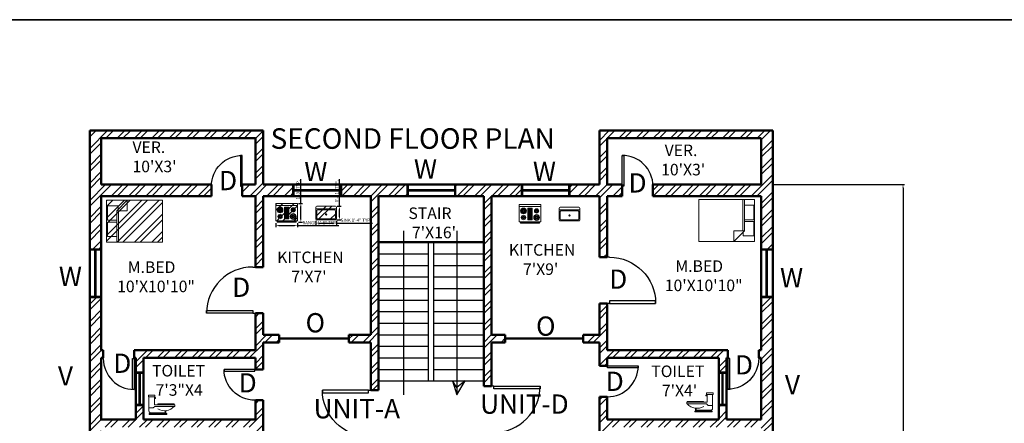
# Model space of a CAD drawing. Units: inches. Extents: x -31842 to -29388, y 18869 to 19743.
# Tile 9 of 12: x -30939 to -30172, y 19429 to 19743. Entities that reach past the tile are written whole.
import ezdxf

# ---------------------------------------------------------------- set-up
doc = ezdxf.new("R2010")
doc.units = ezdxf.units.IN
for name, color, linetype, lineweight in [('A-ANNO-DIMS', 2, 'Continuous', 18), ('A-ANNO-SYMB', 2, 'Continuous', 18), ('A-ANNO-TEXT', 7, 'Continuous', 25), ('A-ANNO-TTLB', 7, 'Continuous', 35), ('A-AREA-IDEN', 3, 'Continuous', 18), ('A-DOOR', 3, 'Continuous', 25), ('A-FLOR-FIXT', 8, 'Continuous', 18), ('A-FLOR-STRS', 7, 'Continuous', 25), ('A-FURN', 8, 'Continuous', 18), ('A-GLAZ', 4, 'Continuous', 25), ('A-WALL', 7, 'Continuous', 50), ('A-WALL-PATT', 8, 'Continuous', 13)]:
    doc.layers.add(name, color=color, linetype=linetype, lineweight=lineweight)
doc.styles.get("Standard").update_dxf_attribs({"font": 'arial.ttf'})
doc.dimstyles.new('ISO-25', dxfattribs={"dimtxt": 2.5, "dimasz": 2.5, "dimexe": 1.25, "dimexo": 0.625, "dimtad": 1, "dimdec": 0, "dimlunit": 3, "dimtxsty": 'Standard', "dimcen": 2.5, "dimadec": 0, "dimazin": 0, "dimtfac": 1, "dimtdec": 0, "dimtmove": 0, "dimatfit": 3, "dimfxl": 1, "dimarcsym": 0})

# ---------------------------------------------------------------- blocks, each defined once
blk = doc.blocks.new('*U8')
for p, q in [((0, 0), (0, -100)), ((750, 0), (750, -100))]:
    blk.add_line(p, q)
blk.add_lwpolyline([(0, 0), (0, 750), (43.75, 750), (43.75, 0)], close=True)
blk.add_arc((0, 0), 750, 0, 90)
blk = doc.blocks.new('Bed - Queen')
for p, q in [((0, -80.00003), (0, 0)), ((0, 0), (59.99999, 0)), ((59.99999, 0), (59.99999, -80.00003)), ((7.99999, -1.2), (28.79998, -1.2)), ((7.99999, -14.4), (7.99999, -1.2)), ((28.79998, -1.2), (28.79998, -14.4)), ((31.19999, -1.2), (51.99999, -1.2)), ((31.19999, -14.4), (31.19999, -1.2)), ((51.99999, -1.2), (51.99999, -16.4)), ((0, -14.4), (44.8, -14.4)), ((44.8, -16.8), (0, -16.8)), ((59.99999, -29.6), (44.8, -14.4)), ((44.8, -14.4), (44.8, -29.6)), ((51.99999, -16.4), (46.79936, -16.4)), ((44.8, -29.6), (59.99999, -29.6)), ((59.99999, -80.00003), (0, -80.00003))]:
    blk.add_line(p, q)
blk = doc.blocks.new('Range-Oven - 30 in top')
for p, q in [((0, -3), (30, -3)), ((12, -6), (18, -6)), ((13, -20), (13, -6)), ((14, -6), (14, -20)), ((15, -20), (15, -6)), ((16, -6), (16, -20)), ((17, -20), (17, -6)), ((6, -24), (6, -25)), ((8, -25), (8, -24)), ((18, -20), (12, -20)), ((22, -25), (22, -24)), ((24, -24), (24, -25))]:
    blk.add_line(p, q)
for points in [[(0, -24), (0, 0), (30, 0), (30, -24)], [(12, -21), (12, -5), (18, -5), (18, -21)], [(2, -26), (2, -25), (28, -25), (28, -26)]]:
    blk.add_lwpolyline(points, close=True)
for centre, radius in [((6, -9), 4), ((6, -9), 3), ((6, -9), 2), ((6, -9), 1), ((24, -9), 3), ((24, -9), 2), ((24, -9), 1), ((6, -18), 3), ((6, -18), 2), ((6, -18), 1), ((24, -18), 4), ((24, -18), 3), ((24, -18), 2), ((24, -18), 1)]:
    blk.add_circle(centre, radius)
blk = doc.blocks.new('Sink-single - 30 in top')
blk.add_line((-15, -3.999996), (15, -3.999996))
for points in [[(-13.5, 0), (13.5, 0)], [(-15, -18.499996), (-15, -1.5)], [(-13.5, -17.499996), (-13.5, -6.499996)], [(-12.5, -5.499996), (12.5, -5.499996)], [(13.5, -6.499996), (13.5, -17.499996)], [(15, -1.5), (15, -18.499996)], [(13.5, -19.999996), (-13.5, -19.999996)], [(12.5, -18.499996), (-12.5, -18.499996)]]:
    blk.add_lwpolyline(points)
for radius in [1, 0.5]:
    blk.add_circle((0, -11.999996), radius)
for centre, radius, start, end in [((-13.5, -1.5), 1.5, 90, 180), ((-12.5, -6.499996), 1, 90, 180), ((12.5, -6.499996), 1, 0, 90), ((13.5, -1.5), 1.5, 0, 90), ((-13.5, -18.499996), 1.5, 180, 270), ((-12.5, -17.499996), 1, 180, 270), ((12.5, -17.499996), 1, 270, 0), ((13.5, -18.499996), 1.5, 270, 0)]:
    blk.add_arc(centre, radius, start, end)
blk = doc.blocks.new('Toilet - side')
for p, q in [((0.5, 5), (0.5, 22)), ((7.5, 22), (7.5, 12)), ((7.5, 21), (9, 21)), ((9, 20), (7.5, 20)), ((9, 21), (9, 20)), ((32.5, 13), (12, 13)), ((12, 13), (12, 12)), ((32.5, 12), (32.5, 13)), ((6, 8), (0.5, 8)), ((22, 2), (2, 2)), ((2, 2), (2, 1)), ((8, 10), (6, 8)), ((7.5, 12), (33, 12)), ((33, 10), (8, 10)), ((21, 4.5), (21, 2)), ((22, 2), (22, 4.5)), ((22, 1), (22, 2)), ((33, 12), (33, 10))]:
    blk.add_line(p, q)
for points in [[(0, 22), (0, 24), (8, 24), (8, 22)], [(1, 0), (1, 1), (23, 1), (23, 0)]]:
    blk.add_lwpolyline(points, close=True)
for centre, radius, start, end in [((3.8, 4.8), 3.26, 175.6013, 237.5288), ((20.3, 20.7), 16.2, 238.1872, 318.7702)]:
    blk.add_arc(centre, radius, start, end)
blk = doc.blocks.new('*D203')
at = {"layer": 'A-ANNO-DIMS', "color": 0, "lineweight": -2, "transparency": 16777216}
for p, q in [((-30351.77, 19614.99), (-30249.67, 19614.99)), ((-30250.92, 19612.49), (-30250.92, 19017.46)), ((-30351.77, 19014.96), (-30249.67, 19014.96))]:
    blk.add_line(p, q, dxfattribs=at)
at = {"layer": 'A-ANNO-DIMS', "color": 0, "transparency": 16777216}
for points in [[(-30251.34, 19612.49), (-30250.5, 19612.49), (-30250.92, 19614.99)], [(-30251.34, 19017.46), (-30250.5, 19017.46), (-30250.92, 19014.96)]]:
    blk.add_solid(points, dxfattribs=at)
at = {"layer": 'Defpoints', "color": 0, "transparency": 16777216}
for p in [(-30352.39, 19614.99), (-30352.39, 19014.96), (-30250.92, 19014.96)]:
    blk.add_point(p, dxfattribs=at)
at = {"layer": 'A-ANNO-DIMS', "color": 0, "transparency": 16777216, "insert": (-30259.72, 19314.97), "char_height": 2.5, "attachment_point": 5, "rotation": 90}
blk.add_mtext("{\\H6.4x;50'}", dxfattribs=at)
blk = doc.blocks.new('WIN-3FT')
for p, q in [((0, 36), (9, 36)), ((4, 0), (4, 36)), ((4.5, 0), (4.5, 36)), ((5, 0), (5, 36)), ((0, 0), (9, 0))]:
    blk.add_line(p, q)
blk = doc.blocks.new('WIN-2FT-B')
for p, q in [((0, 24), (6, 24)), ((2.5, 0), (2.5, 24)), ((3, 0), (3, 24)), ((3.5, 0), (3.5, 24)), ((0, 0), (6, 0))]:
    blk.add_line(p, q)
blk = doc.blocks.new('*D233')
at = {"layer": 'A-ANNO-DIMS', "color": 0, "lineweight": -2, "transparency": 16777216}
for p, q in [((-30739.53, 19584.89), (-30739.53, 19581.71)), ((-30737.03, 19582.96), (-30725, 19582.96)), ((-30722.5, 19584.89), (-30722.5, 19581.71)), ((-30722.5, 19582.96), (-30690.25, 19582.96))]:
    blk.add_line(p, q, dxfattribs=at)
at = {"layer": 'A-ANNO-DIMS', "color": 0, "transparency": 16777216}
for points in [[(-30737.03, 19583.37), (-30737.03, 19582.54), (-30739.53, 19582.96)], [(-30725, 19583.37), (-30725, 19582.54), (-30722.5, 19582.96)]]:
    blk.add_solid(points, dxfattribs=at)
at = {"layer": 'Defpoints', "color": 0, "transparency": 16777216}
for p in [(-30739.53, 19585.51), (-30722.5, 19585.51), (-30722.5, 19582.96)]:
    blk.add_point(p, dxfattribs=at)
at = {"layer": 'A-ANNO-DIMS', "color": 0, "transparency": 16777216, "insert": (-30705.13, 19584.87), "char_height": 2.5, "attachment_point": 5}
blk.add_mtext('RANGE 1\'-5" TYP.', dxfattribs=at)
blk = doc.blocks.new('*D234')
at = {"layer": 'A-ANNO-DIMS', "color": 0, "lineweight": -2, "transparency": 16777216}
for p, q in [((-30719.95, 19600.27), (-30719.95, 19619.02)), ((-30721.88, 19600.27), (-30718.7, 19600.27)), ((-30719.95, 19588.01), (-30719.95, 19597.77)), ((-30721.88, 19585.51), (-30718.7, 19585.51))]:
    blk.add_line(p, q, dxfattribs=at)
at = {"layer": 'A-ANNO-DIMS', "color": 0, "transparency": 16777216}
for points in [[(-30720.36, 19597.77), (-30719.53, 19597.77), (-30719.95, 19600.27)], [(-30720.36, 19588.01), (-30719.53, 19588.01), (-30719.95, 19585.51)]]:
    blk.add_solid(points, dxfattribs=at)
at = {"layer": 'Defpoints', "color": 0, "transparency": 16777216}
for p in [(-30722.5, 19600.27), (-30719.95, 19600.27), (-30722.5, 19585.51)]:
    blk.add_point(p, dxfattribs=at)
at = {"layer": 'A-ANNO-DIMS', "color": 0, "transparency": 16777216, "insert": (-30721.85, 19610.9), "char_height": 2.5, "attachment_point": 5, "rotation": 90}
blk.add_mtext('1\'-3" TYP.', dxfattribs=at)
blk = doc.blocks.new('*D239')
at = {"layer": 'A-ANNO-DIMS', "color": 0, "lineweight": -2, "transparency": 16777216}
for p, q in [((-30708.36, 19586.71), (-30708.36, 19583.67)), ((-30705.86, 19584.92), (-30694.73, 19584.92)), ((-30692.23, 19586.71), (-30692.23, 19583.67)), ((-30692.23, 19584.92), (-30664.13, 19584.92))]:
    blk.add_line(p, q, dxfattribs=at)
at = {"layer": 'A-ANNO-DIMS', "color": 0, "transparency": 16777216}
for points in [[(-30705.86, 19585.33), (-30705.86, 19584.5), (-30708.36, 19584.92)], [(-30694.73, 19585.33), (-30694.73, 19584.5), (-30692.23, 19584.92)]]:
    blk.add_solid(points, dxfattribs=at)
at = {"layer": 'Defpoints', "color": 0, "transparency": 16777216}
for p in [(-30708.36, 19587.34), (-30692.23, 19587.34), (-30692.23, 19584.92)]:
    blk.add_point(p, dxfattribs=at)
at = {"layer": 'A-ANNO-DIMS', "color": 0, "transparency": 16777216, "insert": (-30676.93, 19586.84), "char_height": 2.5, "attachment_point": 5}
blk.add_mtext('SINK 1\'-4" TYP.', dxfattribs=at)
blk = doc.blocks.new('*D240')
at = {"layer": 'A-ANNO-DIMS', "color": 0, "lineweight": -2, "transparency": 16777216}
for p, q in [((-30689.81, 19598.09), (-30689.81, 19619.02)), ((-30691.6, 19598.09), (-30688.56, 19598.09)), ((-30689.81, 19589.84), (-30689.81, 19595.59)), ((-30691.6, 19587.34), (-30688.56, 19587.34))]:
    blk.add_line(p, q, dxfattribs=at)
at = {"layer": 'A-ANNO-DIMS', "color": 0, "transparency": 16777216}
for points in [[(-30690.22, 19595.59), (-30689.39, 19595.59), (-30689.81, 19598.09)], [(-30690.22, 19589.84), (-30689.39, 19589.84), (-30689.81, 19587.34)]]:
    blk.add_solid(points, dxfattribs=at)
at = {"layer": 'Defpoints', "color": 0, "transparency": 16777216}
for p in [(-30692.23, 19598.09), (-30689.81, 19598.09), (-30692.23, 19587.34)]:
    blk.add_point(p, dxfattribs=at)
at = {"layer": 'A-ANNO-DIMS', "color": 0, "transparency": 16777216, "insert": (-30691.71, 19609.81), "char_height": 2.5, "attachment_point": 5, "rotation": 90}
blk.add_mtext('0\'-11" TYP.', dxfattribs=at)

msp = doc.modelspace()

# ---------------------------------------------------------------- hatches: boundary and pattern name
at = {"layer": 'A-WALL-PATT'}
h = msp.add_hatch(dxfattribs=at)
h.set_pattern_fill('ANSI32', color=256)
h.paths.add_polyline_path([(-30352.39, 19656.96), (-30487.39, 19656.96), (-30487.39, 19614.96), (-30510.39, 19614.96), (-30510.39, 19605.96), (-30487.39, 19605.96), (-30487.39, 19558.38), (-30481.39, 19558.38), (-30481.39, 19605.96), (-30469.68, 19605.96), (-30469.68, 19614.96), (-30481.39, 19614.96), (-30481.39, 19650.96), (-30361.39, 19650.96), (-30361.39, 19614.96), (-30445.68, 19614.96), (-30445.68, 19605.96), (-30361.39, 19605.96), (-30361.39, 19564.96), (-30352.39, 19564.96)])
h.paths.add_polyline_path([(-30548.39, 19614.96), (-30599.39, 19614.96), (-30599.39, 19605.96), (-30577.39, 19605.96), (-30577.39, 19457.87), (-30571.39, 19457.87), (-30571.39, 19491.96), (-30560.76, 19491.96), (-30560.76, 19497.96), (-30571.39, 19497.96), (-30571.39, 19605.96), (-30548.39, 19605.96)])
h.paths.add_polyline_path([(-30637.39, 19614.96), (-30688.39, 19614.96), (-30688.39, 19605.96), (-30665.39, 19605.96), (-30665.39, 19497.96), (-30682.48, 19497.96), (-30682.48, 19491.96), (-30665.39, 19491.96), (-30665.39, 19454.79), (-30662.43, 19454.79), (-30659.39, 19454.79), (-30659.39, 19605.96), (-30637.39, 19605.96)])
h.paths.add_polyline_path([(-30789.63, 19614.96), (-30875.39, 19614.96), (-30875.39, 19650.96), (-30755.39, 19650.96), (-30755.39, 19614.96), (-30765.63, 19614.96), (-30765.63, 19605.96), (-30755.39, 19605.96), (-30755.39, 19550.68), (-30749.39, 19550.68), (-30749.39, 19605.96), (-30726.39, 19605.96), (-30726.39, 19614.96), (-30749.39, 19614.96), (-30749.39, 19656.96), (-30884.39, 19656.96), (-30884.39, 19564.96), (-30875.39, 19564.96), (-30875.39, 19605.96), (-30789.63, 19605.96)])
h.paths.add_polyline_path([(-30749.39, 19491.96), (-30736.92, 19491.96), (-30736.92, 19494.96), (-30682.48, 19494.96), (-30682.48, 19497.96), (-30665.39, 19497.96), (-30665.39, 19605.96), (-30688.39, 19605.96), (-30749.39, 19605.96), (-30749.39, 19550.68), (-30755.39, 19550.68), (-30757.34, 19550.71, 0.39722), (-30793.34, 19516.76), (-30757.34, 19516.76), (-30757.34, 19514.65), (-30793.4, 19514.65), (-30793.4, 19516.76), (-30793.34, 19516.76, -0.39722), (-30757.34, 19550.71), (-30755.39, 19550.71), (-30755.39, 19605.96), (-30765.63, 19605.96), (-30765.63, 19613.66), (-30767.03, 19613.66), (-30767.03, 19637.62, 0.397344), (-30789.63, 19613.65), (-30789.63, 19605.96), (-30875.39, 19605.96), (-30875.39, 19564.96), (-30875.39, 19485.96), (-30873.79, 19485.96), (-30873.79, 19479.96), (-30873.79, 19479.35, 0.39722), (-30851.19, 19455.39), (-30851.19, 19479.35), (-30849.79, 19479.35), (-30849.79, 19455.34), (-30851.19, 19455.34), (-30851.19, 19455.39, -0.39722), (-30873.79, 19479.35), (-30873.79, 19479.96), (-30875.39, 19479.96), (-30875.39, 19431.96), (-30848.39, 19431.96), (-30848.39, 19468.96), (-30842.39, 19468.96), (-30842.39, 19479.96), (-30755.39, 19479.96), (-30755.39, 19470.97), (-30749.39, 19470.97)])
h.paths.add_polyline_path([(-30738.39, 19585.51), (-30738.39, 19586.08), (-30736.12, 19586.08), (-30736.12, 19586.65), (-30739.53, 19586.65), (-30739.53, 19600.27), (-30722.5, 19600.27), (-30722.5, 19586.65), (-30725.91, 19586.65), (-30725.91, 19586.08), (-30723.64, 19586.08), (-30723.64, 19585.51)], flags=16)
h.paths.add_polyline_path([(-30737.83, 19590.05, -1), (-30734.42, 19590.05, -1)], flags=16)
h.paths.add_polyline_path([(-30737.26, 19590.05, -1), (-30734.99, 19590.05, -1)], flags=0)
h.paths.add_polyline_path([(-30732.72, 19588.35), (-30732.72, 19597.43), (-30729.31, 19597.43), (-30729.31, 19588.35)], flags=16)
h.paths.add_polyline_path([(-30736.69, 19590.05, -1), (-30735.56, 19590.05, -1)], flags=0)
h.paths.add_polyline_path([(-30732.15, 19588.92), (-30732.15, 19596.86), (-30729.88, 19596.86), (-30729.88, 19588.92)], flags=0)
h.paths.add_polyline_path([(-30728.18, 19590.05, -1), (-30723.64, 19590.05, -1)], flags=0)
h.paths.add_polyline_path([(-30727.61, 19590.05, -1), (-30724.2, 19590.05, -1)], flags=0)
h.paths.add_polyline_path([(-30727.04, 19590.05, -1), (-30724.77, 19590.05, -1)], flags=0)
h.paths.add_polyline_path([(-30726.47, 19590.05, -1), (-30725.34, 19590.05, -1)], flags=0)
h.paths.add_polyline_path([(-30738.39, 19595.16, -1), (-30733.85, 19595.16, -1)], flags=16)
h.paths.add_polyline_path([(-30737.83, 19595.16, -1), (-30734.42, 19595.16, -1)], flags=0)
h.paths.add_polyline_path([(-30737.26, 19595.16, -1), (-30734.99, 19595.16, -1)], flags=0)
h.paths.add_polyline_path([(-30736.69, 19595.16, -1), (-30735.56, 19595.16, -1)], flags=0)
h.paths.add_polyline_path([(-30727.61, 19595.16, -1), (-30724.2, 19595.16, -1)], flags=0)
h.paths.add_polyline_path([(-30727.04, 19595.16, -1), (-30724.77, 19595.16, -1)], flags=0)
h.paths.add_polyline_path([(-30707.55, 19587.34, -0.414214), (-30708.36, 19588.14), (-30708.36, 19597.29, -0.414214), (-30707.55, 19598.09), (-30693.03, 19598.09, -0.414214), (-30692.23, 19597.29), (-30692.23, 19588.14, -0.414214), (-30693.03, 19587.34)], flags=16)
h.paths.add_polyline_path([(-30726.47, 19595.16, -1), (-30725.34, 19595.16, -1)], flags=0)
h.paths.add_polyline_path([(-30827.74, 19570.11), (-30871.22, 19570.11), (-30871.22, 19602.72), (-30827.74, 19602.72)], flags=16)
h.paths.add_polyline_path([(-30707.01, 19588.14, -0.414214), (-30707.55, 19588.68), (-30707.55, 19594.6, -0.414214), (-30707.01, 19595.13), (-30693.57, 19595.13, -0.414214), (-30693.03, 19594.6), (-30693.03, 19588.68, -0.414214), (-30693.57, 19588.14)], flags=0)
h.paths.add_polyline_path([(-30700.02, 19591.64, -1), (-30700.56, 19591.64, -1)], flags=0)
h.paths.add_polyline_path([(-30863.39, 19594.46), (-30863.39, 19574.46), (-30870.57, 19574.46), (-30870.57, 19585.76), (-30863.39, 19585.76), (-30863.39, 19587.07), (-30870.57, 19587.07), (-30870.57, 19598.37), (-30862.31, 19598.37), (-30862.31, 19595.55), (-30855.13, 19602.72), (-30855.13, 19594.46)], flags=0)
h.paths.add_polyline_path([(-30755.39, 19514.65), (-30757.34, 19514.65), (-30793.4, 19514.65), (-30793.4, 19516.76), (-30793.34, 19516.76, -0.39722), (-30757.34, 19550.71), (-30755.39, 19550.71), (-30755.39, 19605.96), (-30765.63, 19605.96), (-30765.63, 19613.66), (-30767.03, 19613.66), (-30767.03, 19637.62, 0.397344), (-30789.63, 19613.65), (-30789.63, 19605.96), (-30875.39, 19605.96), (-30875.39, 19564.96), (-30875.39, 19485.96), (-30873.79, 19485.96), (-30873.79, 19479.96), (-30873.79, 19479.35, 0.39722), (-30851.19, 19455.39), (-30851.19, 19479.35), (-30849.79, 19479.35), (-30849.79, 19479.96), (-30849.79, 19479.96), (-30849.79, 19485.96), (-30755.39, 19485.96)], flags=16)
h.paths.add_polyline_path([(-30665.39, 19605.96), (-30688.39, 19605.96), (-30749.39, 19605.96), (-30749.39, 19550.68), (-30755.39, 19550.68), (-30757.34, 19550.71, 0.39722), (-30793.34, 19516.76), (-30757.34, 19516.76), (-30757.34, 19514.65), (-30755.39, 19514.65), (-30755.39, 19514.68), (-30749.39, 19514.68), (-30749.39, 19497.96), (-30736.92, 19497.96), (-30736.92, 19494.96), (-30682.48, 19494.96), (-30682.48, 19497.96), (-30665.39, 19497.96)], flags=17)
h.paths.add_polyline_path([(-30749.39, 19446.97), (-30755.39, 19446.97), (-30755.39, 19431.96), (-30842.39, 19431.96), (-30842.39, 19442.96), (-30848.39, 19442.96), (-30848.39, 19431.96), (-30875.39, 19431.96), (-30875.39, 19479.96), (-30873.79, 19479.96), (-30873.79, 19482.55), (-30873.79, 19485.96), (-30875.39, 19485.96), (-30875.39, 19526.96), (-30884.39, 19526.96), (-30884.39, 19384.96), (-30875.39, 19384.96), (-30875.39, 19425.96), (-30755.39, 19425.96), (-30755.39, 19414.67), (-30751.3, 19414.67), (-30749.39, 19414.62)])
h.paths.add_polyline_path([(-30848.39, 19468.96), (-30848.39, 19479.96), (-30849.79, 19479.96), (-30849.79, 19479.35), (-30849.79, 19455.34), (-30851.19, 19455.34), (-30851.19, 19455.39, -0.39722), (-30873.79, 19479.35), (-30873.79, 19479.96), (-30875.39, 19479.96), (-30875.39, 19431.96), (-30848.39, 19431.96), (-30848.39, 19442.96)], flags=17)
h.paths.add_polyline_path([(-30659.39, 19407.96), (-30657.22, 19407.96), (-30657.22, 19413.96), (-30659.39, 19413.96), (-30659.39, 19418.79), (-30665.39, 19418.79), (-30665.39, 19305.96), (-30749.39, 19305.96), (-30749.39, 19378.62), (-30755.39, 19378.62), (-30755.39, 19305.96), (-30875.39, 19305.96), (-30875.39, 19346.96), (-30884.39, 19346.96), (-30884.39, 19282.96), (-30875.39, 19282.96), (-30875.39, 19299.96), (-30796.39, 19299.96), (-30796.39, 19286.68), (-30790.39, 19286.68), (-30790.39, 19299.96), (-30659.39, 19299.96)])
h.paths.add_polyline_path([(-30352.39, 19346.96), (-30361.39, 19346.96), (-30361.39, 19305.96), (-30481.39, 19305.96), (-30481.39, 19380.1), (-30487.39, 19380.1), (-30487.39, 19305.96), (-30571.39, 19305.96), (-30571.39, 19421.87), (-30577.39, 19421.87), (-30577.39, 19413.96), (-30579.53, 19413.96), (-30579.53, 19407.96), (-30577.39, 19407.96), (-30577.39, 19299.96), (-30446.39, 19299.96), (-30446.39, 19291.76), (-30440.39, 19291.76), (-30440.39, 19299.96), (-30361.39, 19299.96), (-30361.39, 19282.96), (-30352.39, 19282.96)])
h.paths.add_polyline_path([(-30481.39, 19449.62), (-30484.39, 19449.62), (-30487.39, 19449.62), (-30487.39, 19416.1), (-30481.39, 19416.1), (-30481.39, 19425.96), (-30361.39, 19425.96), (-30361.39, 19384.96), (-30352.39, 19384.96), (-30352.39, 19526.96), (-30361.39, 19526.96), (-30361.39, 19485.96), (-30363.32, 19485.96), (-30363.32, 19479.96), (-30361.39, 19479.96), (-30361.39, 19431.96), (-30388.39, 19431.96), (-30388.39, 19442.96), (-30394.39, 19442.96), (-30394.39, 19431.96), (-30481.39, 19431.96)])
h.paths.add_polyline_path([(-30387.32, 19482.76), (-30387.32, 19485.96), (-30481.39, 19485.96), (-30481.39, 19522.38), (-30487.39, 19522.38), (-30487.39, 19497.96), (-30500.08, 19497.96), (-30500.08, 19491.96), (-30487.39, 19491.96), (-30487.39, 19473.62), (-30481.39, 19473.62), (-30481.39, 19479.96), (-30394.39, 19479.96), (-30394.39, 19468.96), (-30388.39, 19468.96), (-30388.39, 19479.96), (-30387.32, 19479.96)])
h.paths.add_polyline_path([(-30626.04, 19413.96), (-30610.58, 19413.96), (-30610.58, 19407.24), (-30608.81, 19407.24), (-30608.81, 19376.14), (-30610.63, 19376.14), (-30610.63, 19407.96), (-30614.39, 19407.96), (-30614.39, 19173.96), (-30532.79, 19173.96), (-30532.79, 19167.96), (-30532.79, 19166.59), (-30532.79, 19167.96), (-30614.39, 19167.96), (-30614.39, 19023.96), (-30568.89, 19023.96), (-30568.89, 19014.96), (-30666.89, 19014.96), (-30666.89, 19018.96), (-30702.89, 19018.96), (-30702.89, 19019.96), (-30666.89, 19019.96), (-30666.89, 19023.96), (-30620.39, 19023.96), (-30620.39, 19167.96), (-30707.45, 19167.96), (-30707.45, 19166.65, -0.39722), (-30741.49, 19130.57), (-30741.49, 19130.51), (-30743.6, 19130.51), (-30743.6, 19166.65), (-30741.49, 19166.65), (-30741.49, 19130.57, 0.407721), (-30707.48, 19167.96), (-30707.53, 19167.96), (-30707.53, 19173.96), (-30620.39, 19173.96), (-30620.39, 19407.96), (-30626.04, 19407.96), (-30626.04, 19406.62), (-30626.04, 19375.45), (-30627.86, 19375.45), (-30627.86, 19406.62), (-30626.04, 19406.62), (-30626.04, 19407.96), (-30626.04, 19407.96)])
h.paths.add_polyline_path([(-30481.39, 19167.96), (-30478.24, 19167.96), (-30478.24, 19173.96), (-30487.39, 19173.96), (-30496.79, 19173.96), (-30496.79, 19167.96), (-30487.39, 19167.96), (-30487.39, 19023.96), (-30531.89, 19023.96), (-30531.89, 19014.96), (-30449.39, 19014.96), (-30449.39, 19023.96), (-30481.39, 19023.96)])
h.paths.add_polyline_path([(-30322.39, 19173.96), (-30343.77, 19173.96), (-30343.77, 19167.96), (-30328.39, 19167.96), (-30328.39, 19023.96), (-30373.39, 19023.96), (-30373.39, 19076.96), (-30379.39, 19076.96), (-30379.39, 19023.96), (-30411.39, 19023.96), (-30411.39, 19014.96), (-30322.39, 19014.96)])
h.paths.add_polyline_path([(-30367.77, 19173.96), (-30440.39, 19173.96), (-30440.39, 19191.96), (-30446.39, 19191.96), (-30446.39, 19173.96), (-30449.24, 19173.96), (-30449.24, 19167.96), (-30379.39, 19167.96), (-30379.39, 19114.96), (-30373.39, 19114.96), (-30373.39, 19167.96), (-30367.77, 19167.96)])
h.paths.add_polyline_path([(-30857.39, 19167.96), (-30814.74, 19167.96), (-30787.91, 19167.96), (-30787.91, 19173.96), (-30790.39, 19173.96), (-30790.39, 19191.02), (-30796.39, 19191.02), (-30796.39, 19173.96), (-30814.74, 19173.96), (-30871.78, 19173.96), (-30871.78, 19167.96), (-30863.39, 19167.96), (-30863.39, 19114.96), (-30857.39, 19114.96)])
h.paths.add_polyline_path([(-30857.39, 19076.96), (-30863.39, 19076.96), (-30863.39, 19023.96), (-30908.39, 19023.96), (-30908.39, 19167.96), (-30895.78, 19167.96), (-30895.78, 19173.96), (-30914.39, 19173.96), (-30914.39, 19014.96), (-30825.39, 19014.96), (-30825.39, 19023.96), (-30857.39, 19023.96)])
h.paths.add_polyline_path([(-30758.91, 19173.96), (-30743.53, 19173.96), (-30743.53, 19167.96), (-30743.6, 19166.65), (-30741.49, 19166.65), (-30741.49, 19130.51), (-30743.6, 19130.51), (-30743.6, 19166.65), (-30743.6, 19167.96), (-30749.39, 19167.96), (-30749.39, 19023.96), (-30702.89, 19023.96), (-30702.89, 19019.46), (-30666.89, 19019.46), (-30666.89, 19018.96), (-30702.89, 19018.96), (-30702.89, 19014.96), (-30788.39, 19014.96), (-30788.39, 19018.96), (-30824.39, 19018.96), (-30824.39, 19019.96), (-30788.39, 19019.96), (-30788.39, 19023.96), (-30755.39, 19023.96), (-30755.39, 19167.96), (-30758.91, 19167.96), (-30758.91, 19166.97), (-30758.91, 19137.97), (-30760.6, 19137.97), (-30760.6, 19166.97), (-30758.91, 19166.97), (-30758.91, 19167.96), (-30758.91, 19167.96)])
h.paths.add_polyline_path([(-30790.39, 19237.4), (-30796.39, 19237.4), (-30796.39, 19227.96), (-30875.39, 19227.96), (-30875.39, 19244.96), (-30884.39, 19244.96), (-30884.39, 19210.96), (-30875.39, 19210.96), (-30875.39, 19221.96), (-30796.39, 19221.96), (-30796.39, 19215.02), (-30793.87, 19215.02), (-30790.39, 19215.02)])
h.paths.add_polyline_path([(-30352.39, 19244.96), (-30361.39, 19244.96), (-30361.39, 19227.96), (-30440.39, 19227.96), (-30440.39, 19236.96), (-30446.39, 19236.96), (-30446.39, 19215.96), (-30440.39, 19215.96), (-30440.39, 19221.96), (-30361.39, 19221.96), (-30361.39, 19210.96), (-30352.39, 19210.96)])
h.paths.add_polyline_path([(-30788.99, 19602.36), (-30766.36, 19602.36), (-30766.36, 19633.27), (-30788.99, 19633.27)], flags=24)
h.paths.add_polyline_path([(-30871.43, 19460.05), (-30848.8, 19460.05), (-30848.8, 19490.96), (-30871.43, 19490.96)], flags=24)
h.paths.add_polyline_path([(-30778.82, 19519.23), (-30756.18, 19519.23), (-30756.18, 19550.14), (-30778.82, 19550.14)], flags=24)
h.paths.add_polyline_path([(-30741.54, 19533.68), (-30681.86, 19533.68), (-30681.86, 19567.23), (-30741.54, 19567.23)], flags=24)
h.paths.add_polyline_path([(-30866.65, 19526.15), (-30802.54, 19526.15), (-30802.54, 19559.73), (-30866.65, 19559.73)], flags=8)

# ---------------------------------------------------------------- linework, layer by layer
at = {"layer": 'A-ANNO-TTLB'}
msp.add_lwpolyline([(-31842.18, 19743.36), (-29387.67, 19743.36), (-29387.67, 18868.82), (-31842.18, 18868.82)], close=True, dxfattribs=at)
at = {"layer": 'A-FLOR-STRS'}
for p, q in [((-30639.89, 19578.94), (-30639.89, 19451.21)), ((-30598.41, 19578.94), (-30598.41, 19451.21)), ((-30620.39, 19461.96), (-30620.39, 19569.96)), ((-30616.39, 19461.96), (-30616.39, 19569.96)), ((-30659.39, 19560.96), (-30620.39, 19560.96)), ((-30616.39, 19560.96), (-30577.39, 19560.96)), ((-30659.39, 19551.96), (-30620.39, 19551.96)), ((-30616.39, 19551.96), (-30577.39, 19551.96)), ((-30659.39, 19542.96), (-30620.39, 19542.96)), ((-30616.39, 19542.96), (-30577.39, 19542.96)), ((-30659.39, 19533.96), (-30620.39, 19533.96)), ((-30616.39, 19533.96), (-30577.39, 19533.96)), ((-30659.39, 19524.96), (-30620.39, 19524.96)), ((-30616.39, 19524.96), (-30577.39, 19524.96)), ((-30659.39, 19515.96), (-30620.39, 19515.96)), ((-30616.39, 19515.96), (-30577.39, 19515.96)), ((-30659.39, 19506.96), (-30620.39, 19506.96)), ((-30616.39, 19506.96), (-30577.39, 19506.96)), ((-30659.39, 19497.96), (-30620.39, 19497.96)), ((-30616.39, 19497.96), (-30577.39, 19497.96)), ((-30659.39, 19488.96), (-30620.39, 19488.96)), ((-30616.39, 19488.96), (-30577.39, 19488.96)), ((-30659.39, 19479.96), (-30620.39, 19479.96)), ((-30616.39, 19479.96), (-30577.39, 19479.96)), ((-30659.39, 19470.96), (-30620.39, 19470.96)), ((-30616.39, 19470.96), (-30577.39, 19470.96)), ((-30659.39, 19461.96), (-30577.39, 19461.96)), ((-30598.41, 19456.94), (-30601.94, 19461.96)), ((-30601.94, 19461.96), (-30598.41, 19451.21)), ((-30598.41, 19451.21), (-30592, 19461.96)), ((-30592, 19461.96), (-30598.41, 19456.94))]:
    msp.add_line(p, q, dxfattribs=at)
at = {"layer": 'A-GLAZ'}
for p, q in [((-30726.39, 19614.96), (-30726.39, 19605.96)), ((-30688.39, 19614.96), (-30688.39, 19605.96)), ((-30637.39, 19614.96), (-30637.39, 19605.96)), ((-30599.39, 19614.96), (-30599.39, 19605.96)), ((-30548.39, 19614.96), (-30548.39, 19605.96)), ((-30510.39, 19614.96), (-30510.39, 19605.96)), ((-30884.39, 19564.96), (-30875.39, 19564.96)), ((-30361.39, 19564.96), (-30352.39, 19564.96)), ((-30884.39, 19526.96), (-30875.39, 19526.96)), ((-30361.39, 19526.96), (-30352.39, 19526.96)), ((-30848.39, 19468.96), (-30842.39, 19468.96)), ((-30394.39, 19468.96), (-30388.39, 19468.96)), ((-30848.39, 19442.96), (-30842.39, 19442.96)), ((-30394.39, 19442.96), (-30388.39, 19442.96))]:
    msp.add_line(p, q, dxfattribs=at)
at = {"layer": 'A-WALL'}
for p, q in [((-30884.39, 19173.96), (-30884.39, 19656.96)), ((-30884.39, 19656.96), (-30749.39, 19656.96)), ((-30749.39, 19614.96), (-30749.39, 19656.96)), ((-30487.39, 19656.96), (-30487.39, 19614.96)), ((-30487.39, 19656.96), (-30352.39, 19656.96)), ((-30352.39, 19656.96), (-30352.39, 19173.96)), ((-30875.39, 19650.96), (-30755.39, 19650.96)), ((-30875.39, 19614.96), (-30875.39, 19650.96)), ((-30755.39, 19614.96), (-30755.39, 19650.96)), ((-30481.39, 19650.96), (-30481.39, 19614.96)), ((-30481.39, 19650.96), (-30361.39, 19650.96)), ((-30361.39, 19650.96), (-30361.39, 19614.96)), ((-30875.39, 19614.96), (-30789.63, 19614.96)), ((-30789.63, 19614.96), (-30789.63, 19605.96)), ((-30765.63, 19614.96), (-30765.63, 19605.96)), ((-30765.63, 19614.96), (-30755.39, 19614.96)), ((-30749.39, 19614.96), (-30487.39, 19614.96)), ((-30481.39, 19614.96), (-30469.68, 19614.96)), ((-30469.68, 19614.96), (-30469.68, 19605.96)), ((-30445.68, 19614.96), (-30445.68, 19605.96)), ((-30445.68, 19614.96), (-30361.39, 19614.96)), ((-30875.39, 19605.96), (-30789.63, 19605.96)), ((-30875.39, 19485.96), (-30875.39, 19605.96)), ((-30765.63, 19605.96), (-30755.39, 19605.96)), ((-30755.39, 19550.68), (-30755.39, 19605.96)), ((-30749.39, 19605.96), (-30665.39, 19605.96)), ((-30749.39, 19550.68), (-30749.39, 19605.96)), ((-30665.39, 19497.96), (-30665.39, 19605.96)), ((-30659.39, 19605.96), (-30577.39, 19605.96)), ((-30659.39, 19454.79), (-30659.39, 19605.96)), ((-30577.39, 19605.96), (-30577.39, 19457.87)), ((-30571.39, 19605.96), (-30571.39, 19497.96)), ((-30571.39, 19605.96), (-30487.39, 19605.96)), ((-30487.39, 19605.96), (-30487.39, 19558.38)), ((-30481.39, 19605.96), (-30481.39, 19558.38)), ((-30481.39, 19605.96), (-30469.68, 19605.96)), ((-30445.68, 19605.96), (-30361.39, 19605.96)), ((-30361.39, 19605.96), (-30361.39, 19485.96)), ((-30659.39, 19569.96), (-30577.39, 19569.96)), ((-30487.39, 19558.38), (-30481.39, 19558.38)), ((-30755.39, 19550.68), (-30749.39, 19550.68)), ((-30487.39, 19522.38), (-30481.39, 19522.38)), ((-30487.39, 19522.38), (-30487.39, 19497.96)), ((-30481.39, 19522.38), (-30481.39, 19485.96)), ((-30755.39, 19485.96), (-30755.39, 19514.68)), ((-30755.39, 19514.68), (-30749.39, 19514.68)), ((-30749.39, 19497.96), (-30749.39, 19514.68)), ((-30749.39, 19497.96), (-30736.92, 19497.96)), ((-30736.92, 19497.96), (-30736.92, 19491.96)), ((-30682.48, 19497.96), (-30682.48, 19491.96)), ((-30682.48, 19497.96), (-30665.39, 19497.96)), ((-30571.39, 19497.96), (-30560.76, 19497.96)), ((-30560.76, 19497.96), (-30560.76, 19491.96)), ((-30500.08, 19497.96), (-30500.08, 19491.96)), ((-30500.08, 19497.96), (-30487.39, 19497.96)), ((-30749.39, 19491.96), (-30736.92, 19491.96)), ((-30749.39, 19470.97), (-30749.39, 19491.96)), ((-30736.92, 19494.96), (-30682.48, 19494.96)), ((-30682.48, 19491.96), (-30665.39, 19491.96)), ((-30665.39, 19454.79), (-30665.39, 19491.96)), ((-30571.39, 19491.96), (-30560.76, 19491.96)), ((-30571.39, 19491.96), (-30571.39, 19457.87)), ((-30560.76, 19494.96), (-30500.08, 19494.96)), ((-30500.08, 19491.96), (-30487.39, 19491.96)), ((-30487.39, 19491.96), (-30487.39, 19473.62)), ((-30875.39, 19485.96), (-30873.79, 19485.96)), ((-30873.79, 19479.96), (-30873.79, 19485.96)), ((-30849.79, 19479.96), (-30849.79, 19485.96)), ((-30849.79, 19485.96), (-30755.39, 19485.96)), ((-30481.39, 19485.96), (-30387.32, 19485.96)), ((-30387.32, 19479.96), (-30387.32, 19485.96)), ((-30363.32, 19479.96), (-30363.32, 19485.96)), ((-30363.32, 19485.96), (-30361.39, 19485.96)), ((-30875.39, 19479.96), (-30873.79, 19479.96)), ((-30875.39, 19431.96), (-30875.39, 19479.96)), ((-30849.79, 19479.96), (-30848.39, 19479.96)), ((-30848.39, 19431.96), (-30848.39, 19479.96)), ((-30842.39, 19431.96), (-30842.39, 19479.96)), ((-30842.39, 19479.96), (-30755.39, 19479.96)), ((-30755.39, 19470.97), (-30755.39, 19479.96)), ((-30487.39, 19473.62), (-30481.39, 19473.62)), ((-30481.39, 19479.96), (-30394.39, 19479.96)), ((-30481.39, 19479.96), (-30481.39, 19473.62)), ((-30394.39, 19479.96), (-30394.39, 19431.96)), ((-30388.39, 19479.96), (-30388.39, 19431.96)), ((-30388.39, 19479.96), (-30387.32, 19479.96)), ((-30363.32, 19479.96), (-30361.39, 19479.96)), ((-30361.39, 19479.96), (-30361.39, 19431.96)), ((-30755.39, 19470.97), (-30749.39, 19470.97)), ((-30577.39, 19457.87), (-30571.39, 19457.87)), ((-30665.39, 19454.79), (-30659.39, 19454.79)), ((-30487.39, 19449.62), (-30481.39, 19449.62)), ((-30487.39, 19449.62), (-30487.39, 19416.1)), ((-30481.39, 19449.62), (-30481.39, 19431.96)), ((-30755.39, 19431.96), (-30755.39, 19446.97)), ((-30755.39, 19446.97), (-30749.39, 19446.97)), ((-30749.39, 19414.62), (-30749.39, 19446.97)), ((-30875.39, 19431.96), (-30848.39, 19431.96)), ((-30842.39, 19431.96), (-30755.39, 19431.96)), ((-30481.39, 19431.96), (-30394.39, 19431.96)), ((-30388.39, 19431.96), (-30361.39, 19431.96))]:
    msp.add_line(p, q, dxfattribs=at)

# ---------------------------------------------------------------- block references
at = {"layer": 'A-DOOR'}
for p, xscale, yscale, zscale in [((-30765.63, 19613.66), -0.0319999993054766, 0.0319999993054766, 0.0319999993054766), ((-30469.68, 19613.66), 0.0320000000000009, 0.0320000000000009, 0.0320000000000009)]:
    msp.add_blockref('*U8', p, dxfattribs=dict(at, xscale=xscale, yscale=yscale, zscale=zscale))
for p, xscale, yscale, zscale, rotation in [((-30479.59, 19522.38), -0.0480000000000013, 0.0480000000000013, 0.0480000000000013, 270), ((-30757.34, 19514.65), 0.04808324043333, 0.04808324043333, 0.04808324043333, 90.00000000000003), ((-30849.79, 19479.35), 0.0320047223422117, 0.0320047223422117, 0.0320047223422117, 180), ((-30387.32, 19479.56), -0.0320000000000009, 0.0320000000000009, 0.0320000000000009, 180), ((-30481.19, 19473.62), 0.0320000008125469, 0.0320000008125469, 0.0320000008125469, 270), ((-30755.79, 19470.97), -0.0319858042133018, 0.0319858042133018, 0.0319858042133018, 90), ((-30569.59, 19457.87), 0.0479999960937841, 0.0479999960937841, 0.0479999960937841, 270), ((-30667.22, 19454.79), -0.0479286545029492, 0.0479286545029492, 0.0479286545029492, 90)]:
    msp.add_blockref('*U8', p, dxfattribs=dict(at, xscale=xscale, yscale=yscale, zscale=zscale, rotation=rotation))
at = {"layer": 'A-FLOR-FIXT'}
for name, p, xscale, yscale, zscale in [('Range-Oven - 30 in top', (-30739.53, 19600.27), 0.5676462121975467, 0.5676462121975467, 0.5676462121975467), ('Sink-single - 30 in top', (-30700.29, 19598.09), 0.5377581895364227, 0.5377581895364227, 0.5377581895364227), ('Range-Oven - 30 in top', (-30549.93, 19599.49), 0.5676462121975467, 0.5676462121975467, 0.5676462121975467), ('Sink-single - 30 in top', (-30510.69, 19597.32), 0.5377581895364227, 0.5377581895364227, 0.5377581895364227), ('Toilet - side', (-30838.71, 19435.95), 0.6210234921067381, 0.6210234921067381, 0.6210234921067381), ('Toilet - side', (-30398.88, 19437.86), -0.6210234921067381, 0.6210234921067381, 0.6210234921067381)]:
    msp.add_blockref(name, p, dxfattribs=dict(at, xscale=xscale, yscale=yscale, zscale=zscale))
at = {"layer": 'A-FURN', "xscale": 0.5435212084103092, "yscale": 0.5435212084103092, "zscale": 0.5435212084103092}
for p, rotation in [((-30871.22, 19570.11), 90), ((-30366.47, 19603.18), 270)]:
    msp.add_blockref('Bed - Queen', p, dxfattribs=dict(at, rotation=rotation))
at = {"layer": 'A-GLAZ'}
for p, rotation in [((-30725.39, 19614.96), 269.9999999999509), ((-30636.39, 19614.96), 269.9999999999782), ((-30547.39, 19614.96), 269.9999999999727)]:
    msp.add_blockref('WIN-3FT', p, dxfattribs=dict(at, rotation=rotation))
for name, p in [('WIN-3FT', (-30884.39, 19527.96)), ('WIN-3FT', (-30361.39, 19527.96)), ('WIN-2FT-B', (-30848.39, 19443.96)), ('WIN-2FT-B', (-30394.39, 19443.96))]:
    msp.add_blockref(name, p, dxfattribs=at)

# ---------------------------------------------------------------- texts
at = {"layer": 'A-ANNO-SYMB', "char_height": 15, "attachment_point": 1}
for s, insert in [('{W}', (-30631.84, 19634.55)), ('{W}', (-30717.25, 19632.6)), ('{W}', (-30539.19, 19632.79)), ('{D}', (-30783.63, 19625.55)), ('{D}', (-30464.73, 19623.72)), ('{W}', (-30908.43, 19550.89)), ('{W}', (-30346.69, 19549.83)), ('{D}', (-30773.45, 19542.42)), ('{D}', (-30479.78, 19548.76)), ('{O}', (-30716.27, 19514.79)), ('{O}', (-30536.76, 19512.17)), ('{D}', (-30866.06, 19483.24)), ('{D}', (-30381.85, 19481.98)), ('{V}', (-30909.16, 19473.47)), ('{D}', (-30768.37, 19467.97)), ('{D}', (-30482.47, 19469.17)), ('{V}', (-30342.91, 19466.59))]:
    msp.add_mtext_dynamic_manual_height_columns(s, width=971.0743, gutter_width=12.5, heights=[0], dxfattribs=dict(at, insert=insert))
at = {"layer": 'A-ANNO-TEXT', "insert": (-30743.52, 19658.77), "char_height": 16, "attachment_point": 1}
msp.add_mtext_dynamic_manual_height_columns('{SECOND FLOOR PLAN}', width=1195.2515, gutter_width=12.5, heights=[0], dxfattribs=at)
at = {"layer": 'A-AREA-IDEN', "attachment_point": 1}
for s, width, insert, char_height in [("{VER.\\P10'X3'}", 1016.678, (-30851.07, 19648.52), 9), ("{ VER.\\P10'X3'}", 1016.678, (-30439.3, 19646.09), 9), ("{   STAIR\\P    7'X16'}", 1016.678, (-30644.39, 19597.1), 9), ("{KITCHEN\\P    7'X9'}", 1016.678, (-30557.89, 19568.52), 9), ("{KITCHEN\\P    7'X7'}", 1016.678, (-30738.37, 19562.75), 9), ('{   M.BED\\P10\'X10\'10"}', 1016.678, (-30863.03, 19555.1), 9), ('{   M.BED\\P10\'X10\'10"}', 1016.678, (-30436.46, 19555.9), 9), ('{TOILET\\P 7\'3"X4}', 1016.678, (-30835.84, 19474.42), 9), ("{    TOILET\\P       7'X4'}", 1016.678, (-30457.97, 19473.98), 9), ('{UNIT-D}', 971.0743, (-30580.3, 19451.43), 15), ('{UNIT-A}', 971.0743, (-30710.04, 19447.83), 15)]:
    msp.add_mtext_dynamic_manual_height_columns(s, width=width, gutter_width=12.5, heights=[0], dxfattribs=dict(at, insert=insert, char_height=char_height))

# ---------------------------------------------------------------- dimensions: what is measured, and where the dimension line sits
at = {"layer": 'A-ANNO-DIMS'}
for base, p1, p2, text, override, picture, middle in [((-30719.95, 19600.27), (-30722.5, 19585.51), (-30722.5, 19600.27), '<> TYP.', {"dimdec": 1, "dimlfac": 1, "dimrnd": 0, "dimzin": 1, "dimdsep": 46, "dimlunit": 4, "dimfrac": 2}, '*D234', (-30721.85, 19610.9)), ((-30689.8052, 19598.0924), (-30692.2251, 19587.3373), (-30692.2251, 19598.0924), '<> TYP.', {"dimdec": 1, "dimlfac": 1, "dimrnd": 0, "dimzin": 1, "dimdsep": 46, "dimlunit": 4, "dimfrac": 2}, '*D240', (-30691.7066, 19609.808)), ((-30250.92, 19014.96), (-30352.39, 19614.99), (-30352.39, 19014.96), '{\\H6.4x;<>}', {"dimclrd": 0, "dimclre": 0, "dimclrt": 0}, '*D203', (-30259.72, 19314.97))]:
    dim = msp.add_linear_dim(base=base, p1=p1, p2=p2, angle=90, text=text, dimstyle='ISO-25', override=override, dxfattribs=at)
    dim.commit()
    dim.dimension.update_dxf_attribs({"geometry": picture, "text_midpoint": middle})
for base, p1, p2, text, picture, middle in [((-30722.5, 19582.96), (-30739.53, 19585.51), (-30722.5, 19585.51), 'RANGE <> TYP.', '*D233', (-30705.13, 19584.87)), ((-30692.23, 19584.92), (-30708.36, 19587.34), (-30692.23, 19587.34), 'SINK <> TYP.', '*D239', (-30676.93, 19586.84))]:
    dim = msp.add_linear_dim(base=base, p1=p1, p2=p2, text=text, dimstyle='ISO-25', override={"dimdec": 1, "dimlfac": 1, "dimrnd": 0, "dimzin": 1, "dimdsep": 46, "dimlunit": 4, "dimfrac": 2}, dxfattribs=at)
    dim.commit()
    dim.dimension.update_dxf_attribs({"geometry": picture, "text_midpoint": middle})

doc.saveas('drawing.dxf')
